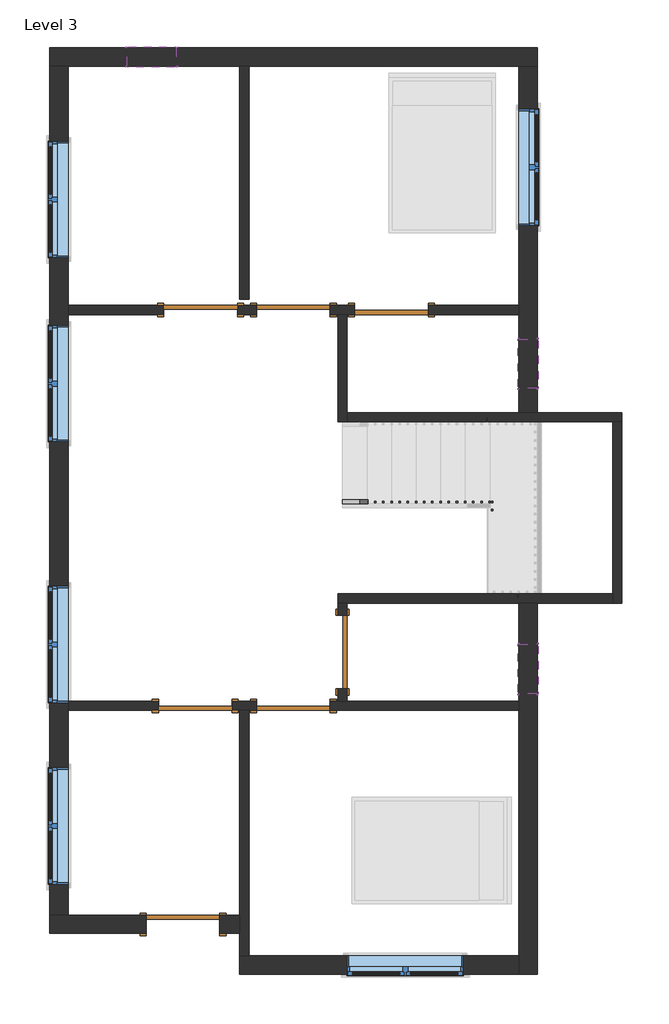
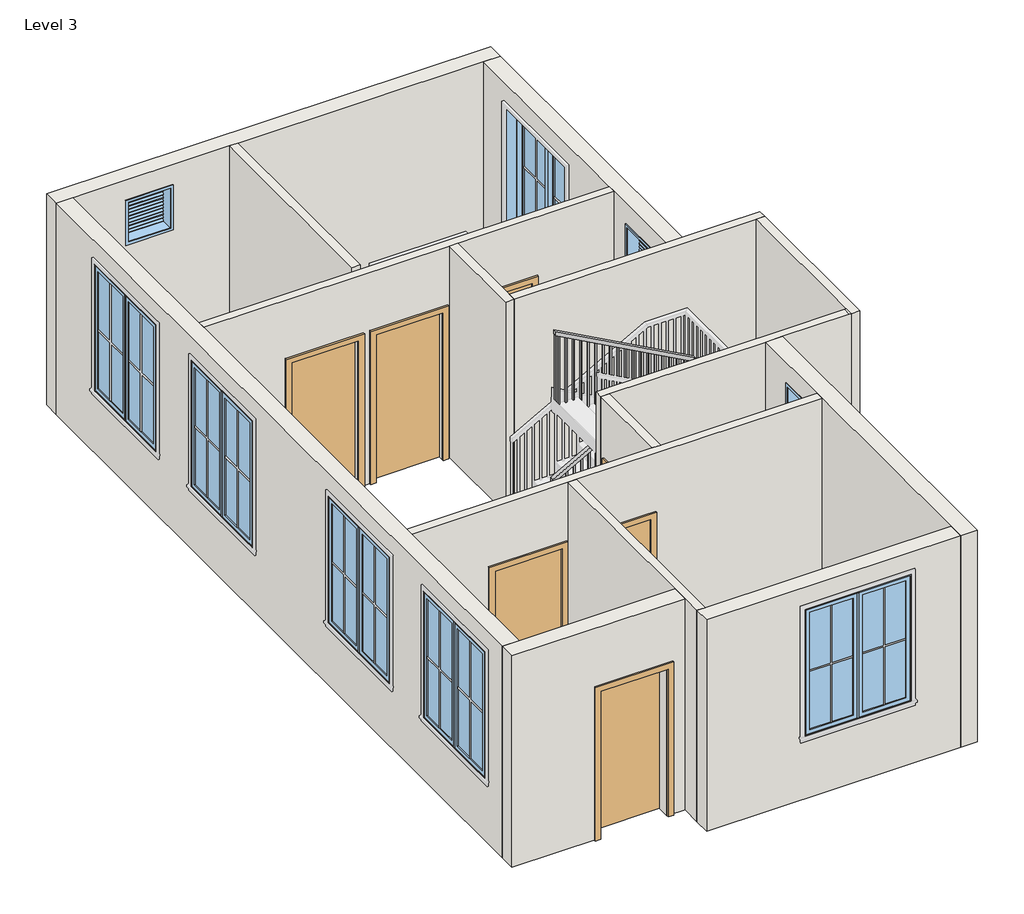
# One storey, part 1 of 2: 15 walls, 9 windows, 7 doors, 1 railing.
"""IFC4 building model written with IfcOpenShell, lengths in millimetres."""

from ifc_helpers import new_model, si_unit, frame, origin, place, context, project, spatial, polyline, outline, extrude, faceted_brep, transform, mapped, element, save
from components import door_e5f9f3c4, door_305aa2a5, door_0ca8825f, window_9ac97e1a, window_f2d8fef0

model = new_model("IFC4")

# Units and contexts
model_context = context("Model", 3, world=origin())
ifc_project = project(units=[si_unit("LENGTHUNIT", "METRE", prefix="MILLI")], contexts=[model_context])

# Site, building, storey
site = spatial("IfcSite", under=ifc_project)
building = spatial("IfcBuilding", under=site)
storey = spatial("IfcBuildingStorey", under=building, Name="Level 3", Elevation=3200.4)

# Doors
placement = place(None, origin())
door_shape = door_e5f9f3c4(model_context)
element("IfcDoor", 1, ObjectType="Single-Flush : 36\" x 84\"", at=placement, inside=storey, context=model_context, shape_type="MappedRepresentation", body=[
    mapped(door_shape, transform((-2929.7888307, 2238.9017201, 3200.4), x_axis=(1.0, 0.0, 0.0), y_axis=(0.0, 1.0, 0.0), z_axis=(0.0, 0.0, 1.0))),
])
element("IfcDoor", 2, ObjectType="Single-Flush : 36\" x 84\"", at=placement, inside=storey, context=model_context, shape_type="MappedRepresentation", body=[
    mapped(door_shape, transform((-558.0638307, 2238.9017201, 3200.4), x_axis=(-1.0, 0.0, 0.0), y_axis=(0.0, -1.0, 0.0), z_axis=(0.0, 0.0, 1.0))),
])
element("IfcDoor", 3, ObjectType="Single-Flush : 36\" x 84\"", at=placement, inside=storey, context=model_context, shape_type="MappedRepresentation", body=[
    mapped(door_shape, transform((-1167.6638307, -2009.2482799, 3200.4), x_axis=(0.0, -1.0, 0.0), y_axis=(1.0, 0.0, 0.0), z_axis=(0.0, 0.0, 1.0))),
])
element("IfcDoor", 4, ObjectType="Single-Flush : 36\" x 84\"", at=placement, inside=storey, context=model_context, shape_type="MappedRepresentation", body=[
    mapped(door_shape, transform((-1777.2638307, -2675.9982799, 3200.4), x_axis=(-1.0, 0.0, 0.0), y_axis=(0.0, -1.0, 0.0), z_axis=(0.0, 0.0, 1.0))),
])
door_2_shape = door_305aa2a5(model_context)
element("IfcDoor", 5, ObjectType="Single-Flush : 36\" x 84\"", at=placement, inside=storey, context=model_context, shape_type="MappedRepresentation", body=[
    mapped(door_2_shape, transform((-1777.2638307, 2238.9017201, 3200.4), x_axis=(-1.0, 0.0, 0.0), y_axis=(0.0, -1.0, 0.0), z_axis=(0.0, 0.0, 1.0))),
])
element("IfcDoor", 6, ObjectType="Single-Flush : 36\" x 84\"", at=placement, inside=storey, context=model_context, shape_type="MappedRepresentation", body=[
    mapped(door_2_shape, transform((-2996.4638307, -2675.9982799, 3200.4), x_axis=(1.0, 0.0, 0.0), y_axis=(0.0, 1.0, 0.0), z_axis=(0.0, 0.0, 1.0))),
])
door_3_shape = door_0ca8825f(model_context)
element("IfcDoor", 7, ObjectType="Single-Flush : 36\" x 84\"", at=placement, inside=storey, context=model_context, shape_type="MappedRepresentation", body=[
    mapped(door_3_shape, transform((-3148.8638307, -5387.4482799, 3200.4), x_axis=(1.0, 0.0, 0.0), y_axis=(0.0, 1.0, 0.0), z_axis=(0.0, 0.0, 1.0))),
])

# Railing
element("IfcRailing", 8, ObjectType="Handrail - Rectangular", at=placement, inside=storey, context=model_context, shape_type="SolidModel", body=[
    faceted_brep([(-1167.6638307, -116.9482799, 4284.1333333), (-1167.6638307, -116.9482799, 4226.0675836), (-1167.6638307, -167.7482799, 4226.0675836), (-1167.6638307, -167.7482799, 4284.1333333), (591.2861693, -116.9482799, 5257.9464821), (642.0861693, -116.9482799, 5228.0052998), (642.0861693, -167.7482799, 5228.0052998), (591.2861693, -167.7482799, 5257.9464821), (591.2861693, -116.9482799, 5300.1333333), (642.0861693, -116.9482799, 5249.3333333), (642.0861693, -167.7482799, 5249.3333333), (591.2861693, -167.7482799, 5300.1333333), (718.2861693, -116.9482799, 5300.1333333), (718.2861693, -116.9482799, 5249.3333333), (667.4861693, -167.7482799, 5249.3333333), (667.4861693, -167.7482799, 5300.1333333), (718.2861693, -218.5482799, 5300.1333333), (667.4861693, -218.5482799, 5300.1333333), (667.4861693, -269.3482799, 5249.3333333), (718.2861693, -269.3482799, 5249.3333333)], [[[0, 1, 2, 3]], [[1, 0, 4, 5]], [[2, 1, 5, 6]], [[3, 2, 6, 7]], [[0, 3, 7, 4]], [[5, 4, 8, 9]], [[6, 5, 9, 10]], [[7, 6, 10, 11]], [[4, 7, 11, 8]], [[9, 8, 12, 13]], [[10, 9, 13, 14]], [[11, 10, 14, 15]], [[8, 11, 15, 12]], [[16, 17, 18, 19]], [[13, 12, 16, 19]], [[14, 13, 19, 18]], [[15, 14, 18, 17]], [[12, 15, 17, 16]]]),
    faceted_brep([(718.2861693, -218.5482799, 5300.1333333), (718.2861693, -269.3482799, 5249.3333333), (667.4861693, -269.3482799, 5249.3333333), (667.4861693, -218.5482799, 5300.1333333), (718.2861693, -218.5482799, 5441.6310502), (667.4861693, -218.5482799, 5411.5403208), (667.4861693, -269.3482799, 5411.5403208), (718.2861693, -269.3482799, 5441.6310502)], [[[0, 1, 2, 3]], [[4, 5, 6, 7]], [[1, 0, 4, 7]], [[2, 1, 7, 6]], [[3, 2, 6, 5]], [[0, 3, 5, 4]]]),
    faceted_brep([(718.2861693, -269.3482799, 5441.6310502), (667.4861693, -269.3482799, 5411.5403208), (667.4861693, -218.5482799, 5411.5403208), (718.2861693, -218.5482799, 5441.6310502), (-1186.7138307, -269.3482799, 6485.4666667), (-1186.7138307, -218.5482799, 6485.4666667), (-1186.7138307, -218.5482799, 6427.5403208), (-1186.7138307, -269.3482799, 6427.5403208)], [[[0, 1, 2, 3]], [[4, 5, 6, 7]], [[1, 0, 4, 7]], [[2, 1, 7, 6]], [[3, 2, 6, 5]], [[0, 3, 5, 4]]]),
    extrude(outline(polyline([(6394.4855263, -1126.3888307), (6404.9238825, -1145.4388307), (5401.7333333, -1145.4388307), (5401.7333333, -1126.3888307), (6394.4855263, -1126.3888307)])), frame((0.0, -253.4732799, 0.0), z_axis=(0.0, 1.0, 0.0), x_axis=(0.0, 0.0, 1.0)), (0.0, 0.0, 1.0), 19.05),
    extrude(outline(polyline([(6338.8142934, -1024.7888307), (6349.2526496, -1043.8388307), (5401.7333333, -1043.8388307), (5401.7333333, -1024.7888307), (6338.8142934, -1024.7888307)])), frame((0.0, -253.4732799, 0.0), z_axis=(0.0, 1.0, 0.0), x_axis=(0.0, 0.0, 1.0)), (0.0, 0.0, 1.0), 19.05),
    extrude(outline(polyline([(6283.1430606, -923.1888307), (6293.5814167, -942.2388307), (5401.7333333, -942.2388307), (5401.7333333, -923.1888307), (6283.1430606, -923.1888307)])), frame((0.0, -253.4732799, 0.0), z_axis=(0.0, 1.0, 0.0), x_axis=(0.0, 0.0, 1.0)), (0.0, 0.0, 1.0), 19.05),
    extrude(outline(polyline([(6227.4718277, -821.5888307), (6237.9101838, -840.6388307), (5232.4, -840.6388307), (5232.4, -821.5888307), (6227.4718277, -821.5888307)])), frame((0.0, -253.4732799, 0.0), z_axis=(0.0, 1.0, 0.0), x_axis=(0.0, 0.0, 1.0)), (0.0, 0.0, 1.0), 19.05),
    extrude(outline(polyline([(6171.8005948, -719.9888307), (6182.238951, -739.0388307), (5232.4, -739.0388307), (5232.4, -719.9888307), (6171.8005948, -719.9888307)])), frame((0.0, -253.4732799, 0.0), z_axis=(0.0, 1.0, 0.0), x_axis=(0.0, 0.0, 1.0)), (0.0, 0.0, 1.0), 19.05),
    extrude(outline(polyline([(6116.1293619, -618.3888307), (6126.5677181, -637.4388307), (5232.4, -637.4388307), (5232.4, -618.3888307), (6116.1293619, -618.3888307)])), frame((0.0, -253.4732799, 0.0), z_axis=(0.0, 1.0, 0.0), x_axis=(0.0, 0.0, 1.0)), (0.0, 0.0, 1.0), 19.05),
    extrude(outline(polyline([(6060.458129, -516.7888307), (6070.8964852, -535.8388307), (5063.0666667, -535.8388307), (5063.0666667, -516.7888307), (6060.458129, -516.7888307)])), frame((0.0, -253.4732799, 0.0), z_axis=(0.0, 1.0, 0.0), x_axis=(0.0, 0.0, 1.0)), (0.0, 0.0, 1.0), 19.05),
    extrude(outline(polyline([(6004.7868962, -415.1888307), (6015.2252523, -434.2388307), (5063.0666667, -434.2388307), (5063.0666667, -415.1888307), (6004.7868962, -415.1888307)])), frame((0.0, -253.4732799, 0.0), z_axis=(0.0, 1.0, 0.0), x_axis=(0.0, 0.0, 1.0)), (0.0, 0.0, 1.0), 19.05),
    extrude(outline(polyline([(5949.1156633, -313.5888307), (5959.5540195, -332.6388307), (5063.0666667, -332.6388307), (5063.0666667, -313.5888307), (5949.1156633, -313.5888307)])), frame((0.0, -253.4732799, 0.0), z_axis=(0.0, 1.0, 0.0), x_axis=(0.0, 0.0, 1.0)), (0.0, 0.0, 1.0), 19.05),
    extrude(outline(polyline([(5893.4444304, -211.9888307), (5903.8827866, -231.0388307), (4893.7333333, -231.0388307), (4893.7333333, -211.9888307), (5893.4444304, -211.9888307)])), frame((0.0, -253.4732799, 0.0), z_axis=(0.0, 1.0, 0.0), x_axis=(0.0, 0.0, 1.0)), (0.0, 0.0, 1.0), 19.05),
    extrude(outline(polyline([(5837.7731975, -110.3888307), (5848.2115537, -129.4388307), (4893.7333333, -129.4388307), (4893.7333333, -110.3888307), (5837.7731975, -110.3888307)])), frame((0.0, -253.4732799, 0.0), z_axis=(0.0, 1.0, 0.0), x_axis=(0.0, 0.0, 1.0)), (0.0, 0.0, 1.0), 19.05),
    extrude(outline(polyline([(5782.1019647, -8.7888307), (5792.5403208, -27.8388307), (4893.7333333, -27.8388307), (4893.7333333, -8.7888307), (5782.1019647, -8.7888307)])), frame((0.0, -253.4732799, 0.0), z_axis=(0.0, 1.0, 0.0), x_axis=(0.0, 0.0, 1.0)), (0.0, 0.0, 1.0), 19.05),
    extrude(outline(polyline([(5726.4307318, 92.8111693), (5736.8690879, 73.7611693), (4724.4, 73.7611693), (4724.4, 92.8111693), (5726.4307318, 92.8111693)])), frame((0.0, -253.4732799, 0.0), z_axis=(0.0, 1.0, 0.0), x_axis=(0.0, 0.0, 1.0)), (0.0, 0.0, 1.0), 19.05),
    extrude(outline(polyline([(5670.7594989, 194.4111693), (5681.1978551, 175.3611693), (4724.4, 175.3611693), (4724.4, 194.4111693), (5670.7594989, 194.4111693)])), frame((0.0, -253.4732799, 0.0), z_axis=(0.0, 1.0, 0.0), x_axis=(0.0, 0.0, 1.0)), (0.0, 0.0, 1.0), 19.05),
    extrude(outline(polyline([(5615.088266, 296.0111693), (5625.5266222, 276.9611693), (4724.4, 276.9611693), (4724.4, 296.0111693), (5615.088266, 296.0111693)])), frame((0.0, -253.4732799, 0.0), z_axis=(0.0, 1.0, 0.0), x_axis=(0.0, 0.0, 1.0)), (0.0, 0.0, 1.0), 19.05),
    extrude(outline(polyline([(5559.4170332, 397.6111693), (5569.8553893, 378.5611693), (4555.0666667, 378.5611693), (4555.0666667, 397.6111693), (5559.4170332, 397.6111693)])), frame((0.0, -253.4732799, 0.0), z_axis=(0.0, 1.0, 0.0), x_axis=(0.0, 0.0, 1.0)), (0.0, 0.0, 1.0), 19.05),
    extrude(outline(polyline([(5503.7458003, 499.2111693), (5514.1841564, 480.1611693), (4555.0666667, 480.1611693), (4555.0666667, 499.2111693), (5503.7458003, 499.2111693)])), frame((0.0, -253.4732799, 0.0), z_axis=(0.0, 1.0, 0.0), x_axis=(0.0, 0.0, 1.0)), (0.0, 0.0, 1.0), 19.05),
    extrude(outline(polyline([(5448.0745674, 600.8111693), (5458.5129236, 581.7611693), (4555.0666667, 581.7611693), (4555.0666667, 600.8111693), (5448.0745674, 600.8111693)])), frame((0.0, -253.4732799, 0.0), z_axis=(0.0, 1.0, 0.0), x_axis=(0.0, 0.0, 1.0)), (0.0, 0.0, 1.0), 19.05),
    extrude(outline(polyline([(651.6111693, -151.8732799), (651.6111693, -132.8232799), (670.6611693, -132.8232799), (670.6611693, -151.8732799), (651.6111693, -151.8732799)])), frame((0.0, 0.0, 4216.4), z_axis=(0.0, 0.0, 1.0), x_axis=(1.0, 0.0, 0.0)), (0.0, 0.0, 1.0), 1032.9333333),
    extrude(outline(polyline([(5187.5762341, 569.0611693), (5177.0295213, 550.0111693), (4216.4, 550.0111693), (4216.4, 569.0611693), (5187.5762341, 569.0611693)])), frame((0.0, -151.8732799, 0.0), z_axis=(0.0, 1.0, 0.0), x_axis=(0.0, 0.0, 1.0)), (0.0, 0.0, 1.0), 19.05),
    extrude(outline(polyline([(5131.3270991, 467.4611693), (5120.7803863, 448.4111693), (4216.4, 448.4111693), (4216.4, 467.4611693), (5131.3270991, 467.4611693)])), frame((0.0, -151.8732799, 0.0), z_axis=(0.0, 1.0, 0.0), x_axis=(0.0, 0.0, 1.0)), (0.0, 0.0, 1.0), 19.05),
    extrude(outline(polyline([(5075.0779642, 365.8611693), (5064.5312514, 346.8111693), (4047.0666667, 346.8111693), (4047.0666667, 365.8611693), (5075.0779642, 365.8611693)])), frame((0.0, -151.8732799, 0.0), z_axis=(0.0, 1.0, 0.0), x_axis=(0.0, 0.0, 1.0)), (0.0, 0.0, 1.0), 19.05),
    extrude(outline(polyline([(5018.8288292, 264.2611693), (5008.2821164, 245.2111693), (4047.0666667, 245.2111693), (4047.0666667, 264.2611693), (5018.8288292, 264.2611693)])), frame((0.0, -151.8732799, 0.0), z_axis=(0.0, 1.0, 0.0), x_axis=(0.0, 0.0, 1.0)), (0.0, 0.0, 1.0), 19.05),
    extrude(outline(polyline([(4962.5796943, 162.6611693), (4952.0329815, 143.6111693), (4047.0666667, 143.6111693), (4047.0666667, 162.6611693), (4962.5796943, 162.6611693)])), frame((0.0, -151.8732799, 0.0), z_axis=(0.0, 1.0, 0.0), x_axis=(0.0, 0.0, 1.0)), (0.0, 0.0, 1.0), 19.05),
    extrude(outline(polyline([(4906.3305593, 61.0611693), (4895.7838465, 42.0111693), (3877.7333333, 42.0111693), (3877.7333333, 61.0611693), (4906.3305593, 61.0611693)])), frame((0.0, -151.8732799, 0.0), z_axis=(0.0, 1.0, 0.0), x_axis=(0.0, 0.0, 1.0)), (0.0, 0.0, 1.0), 19.05),
    extrude(outline(polyline([(4850.0814244, -40.5388307), (4839.5347116, -59.5888307), (3877.7333333, -59.5888307), (3877.7333333, -40.5388307), (4850.0814244, -40.5388307)])), frame((0.0, -151.8732799, 0.0), z_axis=(0.0, 1.0, 0.0), x_axis=(0.0, 0.0, 1.0)), (0.0, 0.0, 1.0), 19.05),
    extrude(outline(polyline([(4793.8322895, -142.1388307), (4783.2855766, -161.1888307), (3877.7333333, -161.1888307), (3877.7333333, -142.1388307), (4793.8322895, -142.1388307)])), frame((0.0, -151.8732799, 0.0), z_axis=(0.0, 1.0, 0.0), x_axis=(0.0, 0.0, 1.0)), (0.0, 0.0, 1.0), 19.05),
    extrude(outline(polyline([(4737.5831545, -243.7388307), (4727.0364417, -262.7888307), (3708.4, -262.7888307), (3708.4, -243.7388307), (4737.5831545, -243.7388307)])), frame((0.0, -151.8732799, 0.0), z_axis=(0.0, 1.0, 0.0), x_axis=(0.0, 0.0, 1.0)), (0.0, 0.0, 1.0), 19.05),
    extrude(outline(polyline([(4681.3340196, -345.3388307), (4670.7873068, -364.3888307), (3708.4, -364.3888307), (3708.4, -345.3388307), (4681.3340196, -345.3388307)])), frame((0.0, -151.8732799, 0.0), z_axis=(0.0, 1.0, 0.0), x_axis=(0.0, 0.0, 1.0)), (0.0, 0.0, 1.0), 19.05),
    extrude(outline(polyline([(4625.0848846, -446.9388307), (4614.5381718, -465.9888307), (3708.4, -465.9888307), (3708.4, -446.9388307), (4625.0848846, -446.9388307)])), frame((0.0, -151.8732799, 0.0), z_axis=(0.0, 1.0, 0.0), x_axis=(0.0, 0.0, 1.0)), (0.0, 0.0, 1.0), 19.05),
    extrude(outline(polyline([(4568.8357497, -548.5388307), (4558.2890369, -567.5888307), (3539.0666667, -567.5888307), (3539.0666667, -548.5388307), (4568.8357497, -548.5388307)])), frame((0.0, -151.8732799, 0.0), z_axis=(0.0, 1.0, 0.0), x_axis=(0.0, 0.0, 1.0)), (0.0, 0.0, 1.0), 19.05),
    extrude(outline(polyline([(4512.5866147, -650.1388307), (4502.0399019, -669.1888307), (3539.0666667, -669.1888307), (3539.0666667, -650.1388307), (4512.5866147, -650.1388307)])), frame((0.0, -151.8732799, 0.0), z_axis=(0.0, 1.0, 0.0), x_axis=(0.0, 0.0, 1.0)), (0.0, 0.0, 1.0), 19.05),
    extrude(outline(polyline([(4456.3374798, -751.7388307), (4445.790767, -770.7888307), (3539.0666667, -770.7888307), (3539.0666667, -751.7388307), (4456.3374798, -751.7388307)])), frame((0.0, -151.8732799, 0.0), z_axis=(0.0, 1.0, 0.0), x_axis=(0.0, 0.0, 1.0)), (0.0, 0.0, 1.0), 19.05),
    extrude(outline(polyline([(4400.0883448, -853.3388307), (4389.541632, -872.3888307), (3369.7333333, -872.3888307), (3369.7333333, -853.3388307), (4400.0883448, -853.3388307)])), frame((0.0, -151.8732799, 0.0), z_axis=(0.0, 1.0, 0.0), x_axis=(0.0, 0.0, 1.0)), (0.0, 0.0, 1.0), 19.05),
    extrude(outline(polyline([(4343.8392099, -954.9388307), (4333.2924971, -973.9888307), (3369.7333333, -973.9888307), (3369.7333333, -954.9388307), (4343.8392099, -954.9388307)])), frame((0.0, -151.8732799, 0.0), z_axis=(0.0, 1.0, 0.0), x_axis=(0.0, 0.0, 1.0)), (0.0, 0.0, 1.0), 19.05),
    extrude(outline(polyline([(4287.5900749, -1056.5388307), (4277.0433621, -1075.5888307), (3369.7333333, -1075.5888307), (3369.7333333, -1056.5388307), (4287.5900749, -1056.5388307)])), frame((0.0, -151.8732799, 0.0), z_axis=(0.0, 1.0, 0.0), x_axis=(0.0, 0.0, 1.0)), (0.0, 0.0, 1.0), 19.05),
    extrude(outline(polyline([(683.3611693, -234.4232799), (702.4111693, -234.4232799), (702.4111693, -253.4732799), (683.3611693, -253.4732799), (683.3611693, -234.4232799)])), frame((0.0, 0.0, 4385.7333333), z_axis=(0.0, 0.0, 1.0), x_axis=(1.0, 0.0, 0.0)), (0.0, 0.0, 1.0), 863.6),
    extrude(outline(polyline([(683.3611693, -151.8732799), (683.3611693, -132.8232799), (702.4111693, -132.8232799), (702.4111693, -151.8732799), (683.3611693, -151.8732799)])), frame((0.0, 0.0, 4385.7333333), z_axis=(0.0, 0.0, 1.0), x_axis=(1.0, 0.0, 0.0)), (0.0, 0.0, 1.0), 863.6),
    extrude(outline(polyline([(6417.1019647, -1167.6638307), (6427.5403208, -1186.7138307), (5401.7333333, -1186.7138307), (5401.7333333, -1167.6638307), (6417.1019647, -1167.6638307)])), frame((0.0, -253.4732799, 0.0), z_axis=(0.0, 1.0, 0.0), x_axis=(0.0, 0.0, 1.0)), (0.0, 0.0, 1.0), 19.05),
    extrude(outline(polyline([(4236.6142964, -1148.6138307), (4226.0675836, -1167.6638307), (3369.7333333, -1167.6638307), (3369.7333333, -1148.6138307), (4236.6142964, -1148.6138307)])), frame((0.0, -151.8732799, 0.0), z_axis=(0.0, 1.0, 0.0), x_axis=(0.0, 0.0, 1.0)), (0.0, 0.0, 1.0), 19.05),
])

# Walls
element("IfcWall", 9, ObjectType="WALL 4.5\"", at=placement, inside=storey, context=model_context, shape_type="SweptSolid", body=[
    extrude(outline(polyline([(-2444.0138307, 2372.2517201), (-2444.0138307, 5267.8517201), (-2329.7138307, 5267.8517201), (-2329.7138307, 2372.2517201), (-2444.0138307, 2372.2517201)])), frame((0.0, 0.0, 3200.4), z_axis=(0.0, 0.0, 1.0), x_axis=(1.0, 0.0, 0.0)), (0.0, 0.0, 1.0), 3048.0),
])
element("IfcWall", 10, ObjectType="WALL 4.5\"", at=placement, inside=storey, context=model_context, shape_type="Brep", body=[
    faceted_brep([(-1320.0638307, 2181.7517201, 3200.4), (-1224.8138307, 2181.7517201, 3200.4), (-1110.5138307, 2181.7517201, 3200.4), (-1015.2638307, 2181.7517201, 3200.4), (-1015.2638307, 2181.7517201, 5334.0), (-100.8638307, 2181.7517201, 5334.0), (-100.8638307, 2181.7517201, 3200.4), (1023.0861693, 2181.7517201, 3200.4), (1023.0861693, 2181.7517201, 6248.4), (-1110.5138307, 2181.7517201, 6248.4), (-1224.8138307, 2181.7517201, 6248.4), (-4577.6138307, 2181.7517201, 6248.4), (-4577.6138307, 2181.7517201, 3200.4), (-3386.9888307, 2181.7517201, 3200.4), (-3386.9888307, 2181.7517201, 5334.0), (-2472.5888307, 2181.7517201, 5334.0), (-2472.5888307, 2181.7517201, 3200.4), (-2234.4638307, 2181.7517201, 3200.4), (-2234.4638307, 2181.7517201, 5334.0), (-1320.0638307, 2181.7517201, 5334.0), (-1015.2638307, 2296.0517201, 5334.0), (-1015.2638307, 2296.0517201, 3200.4), (-1320.0638307, 2296.0517201, 3200.4), (-1320.0638307, 2296.0517201, 5334.0), (-2234.4638307, 2296.0517201, 5334.0), (-2234.4638307, 2296.0517201, 3200.4), (-2472.5888307, 2296.0517201, 3200.4), (-2472.5888307, 2296.0517201, 5334.0), (-3386.9888307, 2296.0517201, 5334.0), (-3386.9888307, 2296.0517201, 3200.4), (-4577.6138307, 2296.0517201, 3200.4), (-4577.6138307, 2296.0517201, 6248.4), (1023.0861693, 2296.0517201, 6248.4), (1023.0861693, 2296.0517201, 3200.4), (-100.8638307, 2296.0517201, 3200.4), (-100.8638307, 2296.0517201, 5334.0)], [[[0, 1, 2, 3, 4, 5, 6, 7, 8, 9, 10, 11, 12, 13, 14, 15, 16, 17, 18, 19]], [[20, 21, 22, 23, 24, 25, 26, 27, 28, 29, 30, 31, 32, 33, 34, 35]], [[13, 12, 30, 29]], [[26, 25, 17, 16]], [[34, 33, 7, 6]], [[22, 21, 3, 2, 1, 0]], [[8, 7, 33, 32]], [[12, 11, 31, 30]], [[27, 26, 16, 15]], [[28, 27, 15, 14]], [[29, 28, 14, 13]], [[18, 17, 25, 24]], [[19, 18, 24, 23]], [[0, 19, 23, 22]], [[4, 3, 21, 20]], [[5, 4, 20, 35]], [[6, 5, 35, 34]], [[11, 10, 9, 8, 32, 31]]]),
])
element("IfcWall", 11, ObjectType="WALL 4.5\"", at=placement, inside=storey, context=model_context, shape_type="Brep", body=[
    faceted_brep([(-1224.8138307, 2181.7517201, 3200.4), (-1224.8138307, 848.2517201, 3200.4), (-1224.8138307, 848.2517201, 6248.4), (-1224.8138307, 2181.7517201, 6248.4), (-1110.5138307, 2181.7517201, 3200.4), (-1110.5138307, 2181.7517201, 6248.4), (-1110.5138307, 962.5517201, 6248.4), (-1110.5138307, 848.2517201, 6248.4), (-1110.5138307, 848.2517201, 3200.4), (-1110.5138307, 962.5517201, 3200.4)], [[[0, 1, 2, 3]], [[4, 5, 6, 7, 8, 9]], [[1, 0, 4, 9, 8]], [[0, 3, 5, 4]], [[2, 1, 8, 7]], [[3, 2, 7, 6, 5]]]),
])
element("IfcWall", 12, ObjectType="WALL 4.5\"", at=placement, inside=storey, context=model_context, shape_type="Brep", body=[
    faceted_brep([(-1110.5138307, 848.2517201, 3200.4), (2191.4861693, 848.2517201, 3200.4), (2305.7861693, 848.2517201, 3200.4), (2305.7861693, 848.2517201, 6248.4), (2191.4861693, 848.2517201, 6248.4), (-1110.5138307, 848.2517201, 6248.4), (-1110.5138307, 962.5517201, 3200.4), (-1110.5138307, 962.5517201, 6248.4), (1023.0861693, 962.5517201, 6248.4), (1251.6861693, 962.5517201, 6248.4), (2305.7861693, 962.5517201, 6248.4), (2305.7861693, 962.5517201, 3200.4), (1251.6861693, 962.5517201, 3200.4), (1023.0861693, 962.5517201, 3200.4)], [[[0, 1, 2, 3, 4, 5]], [[6, 7, 8, 9, 10, 11, 12, 13]], [[2, 1, 0, 6, 13, 12, 11]], [[5, 4, 3, 10, 9, 8, 7]], [[0, 5, 7, 6]], [[3, 2, 11, 10]]]),
])
element("IfcWall", 13, ObjectType="WALL 4.5\"", at=placement, inside=storey, context=model_context, shape_type="Brep", body=[
    faceted_brep([(2191.4861693, 848.2517201, 3200.4), (2191.4861693, -1285.3482799, 3200.4), (2191.4861693, -1399.6482799, 3200.4), (2191.4861693, -1399.6482799, 6248.4), (2191.4861693, -1285.3482799, 6248.4), (2191.4861693, 848.2517201, 6248.4), (2305.7861693, 848.2517201, 3200.4), (2305.7861693, 848.2517201, 6248.4), (2305.7861693, -1399.6482799, 6248.4), (2305.7861693, -1399.6482799, 3200.4)], [[[0, 1, 2, 3, 4, 5]], [[6, 7, 8, 9]], [[2, 1, 0, 6, 9]], [[5, 4, 3, 8, 7]], [[0, 5, 7, 6]], [[3, 2, 9, 8]]]),
])
element("IfcWall", 14, ObjectType="WALL 4.5\"", at=placement, inside=storey, context=model_context, shape_type="Brep", body=[
    faceted_brep([(2191.4861693, -1285.3482799, 3200.4), (-1224.8138307, -1285.3482799, 3200.4), (-1224.8138307, -1285.3482799, 6248.4), (-881.9138307, -1285.3482799, 6248.4), (1251.6861693, -1285.3482799, 6248.4), (2166.0861693, -1285.3482799, 6248.4), (2191.4861693, -1285.3482799, 6248.4), (2191.4861693, -1399.6482799, 3200.4), (2191.4861693, -1399.6482799, 6248.4), (2166.0861693, -1399.6482799, 6248.4), (1251.6861693, -1399.6482799, 6248.4), (1023.0861693, -1399.6482799, 6248.4), (-1110.5138307, -1399.6482799, 6248.4), (-1224.8138307, -1399.6482799, 6248.4), (-1224.8138307, -1399.6482799, 3200.4), (-1110.5138307, -1399.6482799, 3200.4), (1023.0861693, -1399.6482799, 3200.4), (1251.6861693, -1399.6482799, 3200.4)], [[[0, 1, 2, 3, 4, 5, 6]], [[7, 8, 9, 10, 11, 12, 13, 14, 15, 16, 17]], [[1, 0, 7, 17, 16, 15, 14]], [[0, 6, 8, 7]], [[2, 1, 14, 13]], [[6, 5, 9, 8]], [[5, 4, 3, 2, 13, 12, 11, 10, 9]]]),
])
element("IfcWall", 15, ObjectType="WALL 4.5\"", at=placement, inside=storey, context=model_context, shape_type="SweptSolid", body=[
    extrude(outline(polyline([(-2466.4482799, 5334.0), (-2466.4482799, 3200.4), (-2618.8482799, 3200.4), (-2618.8482799, 6248.4), (-1399.6482799, 6248.4), (-1399.6482799, 3200.4), (-1552.0482799, 3200.4), (-1552.0482799, 5334.0), (-2466.4482799, 5334.0)])), frame((-1224.8138307, 0.0, 0.0), z_axis=(1.0, 0.0, 0.0), x_axis=(0.0, 1.0, 0.0)), (0.0, 0.0, 1.0), 114.3),
])
element("IfcWall", 16, ObjectType="WALL 4.5\"", at=placement, inside=storey, context=model_context, shape_type="Brep", body=[
    faceted_brep([(-2234.4638307, -2618.8482799, 3200.4), (-2539.2638307, -2618.8482799, 3200.4), (-2539.2638307, -2618.8482799, 5334.0), (-3453.6638307, -2618.8482799, 5334.0), (-3453.6638307, -2618.8482799, 3200.4), (-4577.6138307, -2618.8482799, 3200.4), (-4577.6138307, -2618.8482799, 6248.4), (-1224.8138307, -2618.8482799, 6248.4), (-1110.5138307, -2618.8482799, 6248.4), (1023.0861693, -2618.8482799, 6248.4), (1023.0861693, -2618.8482799, 3200.4), (-1110.5138307, -2618.8482799, 3200.4), (-1224.8138307, -2618.8482799, 3200.4), (-1320.0638307, -2618.8482799, 3200.4), (-1320.0638307, -2618.8482799, 5334.0), (-2234.4638307, -2618.8482799, 5334.0), (-2539.2638307, -2733.1482799, 5334.0), (-2539.2638307, -2733.1482799, 3200.4), (-2444.0138307, -2733.1482799, 3200.4), (-2329.7138307, -2733.1482799, 3200.4), (-2234.4638307, -2733.1482799, 3200.4), (-2234.4638307, -2733.1482799, 5334.0), (-1320.0638307, -2733.1482799, 5334.0), (-1320.0638307, -2733.1482799, 3200.4), (1023.0861693, -2733.1482799, 3200.4), (1023.0861693, -2733.1482799, 6248.4), (-2329.7138307, -2733.1482799, 6248.4), (-2444.0138307, -2733.1482799, 6248.4), (-4577.6138307, -2733.1482799, 6248.4), (-4577.6138307, -2733.1482799, 3200.4), (-3453.6638307, -2733.1482799, 3200.4), (-3453.6638307, -2733.1482799, 5334.0)], [[[0, 1, 2, 3, 4, 5, 6, 7, 8, 9, 10, 11, 12, 13, 14, 15]], [[16, 17, 18, 19, 20, 21, 22, 23, 24, 25, 26, 27, 28, 29, 30, 31]], [[13, 12, 11, 10, 24, 23]], [[30, 29, 5, 4]], [[20, 19, 18, 17, 1, 0]], [[10, 9, 25, 24]], [[6, 5, 29, 28]], [[21, 20, 0, 15]], [[22, 21, 15, 14]], [[23, 22, 14, 13]], [[2, 1, 17, 16]], [[3, 2, 16, 31]], [[4, 3, 31, 30]], [[9, 8, 7, 6, 28, 27, 26, 25]]]),
])
element("IfcWall", 17, ObjectType="WALL 4.5\"", at=placement, inside=storey, context=model_context, shape_type="Brep", body=[
    faceted_brep([(-2329.7138307, -5781.1482799, 3200.4), (-2329.7138307, -2733.1482799, 3200.4), (-2329.7138307, -2733.1482799, 6248.4), (-2329.7138307, -5781.1482799, 6248.4), (-2444.0138307, -5781.1482799, 3200.4), (-2444.0138307, -5781.1482799, 6248.4), (-2444.0138307, -5501.7482799, 6248.4), (-2444.0138307, -5273.1482799, 6248.4), (-2444.0138307, -2733.1482799, 6248.4), (-2444.0138307, -2733.1482799, 3200.4), (-2444.0138307, -5273.1482799, 3200.4), (-2444.0138307, -5501.7482799, 3200.4)], [[[0, 1, 2, 3]], [[4, 5, 6, 7, 8, 9, 10, 11]], [[1, 0, 4, 11, 10, 9]], [[0, 3, 5, 4]], [[2, 1, 9, 8]], [[3, 2, 8, 7, 6, 5]]]),
])
element("IfcWall", 18, ObjectType="WALL 9\"", at=placement, inside=storey, context=model_context, shape_type="Brep", body=[
    faceted_brep([(-4806.2138307, 5267.8517201, 3200.4), (-4577.6138307, 5267.8517201, 3200.4), (-2444.0138307, 5267.8517201, 3200.4), (-2329.7138307, 5267.8517201, 3200.4), (1023.0861693, 5267.8517201, 3200.4), (1251.6861693, 5267.8517201, 3200.4), (1251.6861693, 5267.8517201, 6248.4), (1023.0861693, 5267.8517201, 6248.4), (-2329.7138307, 5267.8517201, 6248.4), (-2444.0138307, 5267.8517201, 6248.4), (-4577.6138307, 5267.8517201, 6248.4), (-4806.2138307, 5267.8517201, 6248.4), (-3844.1888307, 5267.8517201, 5943.6), (-3234.5888307, 5267.8517201, 5943.6), (-3234.5888307, 5267.8517201, 5334.0), (-3844.1888307, 5267.8517201, 5334.0), (-4806.2138307, 5496.4517201, 3200.4), (-4806.2138307, 5496.4517201, 6248.4), (1251.6861693, 5496.4517201, 6248.4), (1251.6861693, 5496.4517201, 3200.4), (-3844.1888307, 5496.4517201, 5943.6), (-3844.1888307, 5496.4517201, 5334.0), (-3234.5888307, 5496.4517201, 5334.0), (-3234.5888307, 5496.4517201, 5943.6)], [[[0, 1, 2, 3, 4, 5, 6, 7, 8, 9, 10, 11], [12, 13, 14, 15]], [[16, 17, 18, 19], [20, 21, 22, 23]], [[5, 4, 3, 2, 1, 0, 16, 19]], [[6, 5, 19, 18]], [[0, 11, 17, 16]], [[21, 20, 12, 15]], [[22, 21, 15, 14]], [[23, 22, 14, 13]], [[20, 23, 13, 12]], [[11, 10, 9, 8, 7, 6, 18, 17]]]),
])
element("IfcWall", 19, ObjectType="WALL 9\"", at=placement, inside=storey, context=model_context, shape_type="Brep", body=[
    faceted_brep([(1023.0861693, 5267.8517201, 3200.4), (1023.0861693, 2296.0517201, 3200.4), (1023.0861693, 2181.7517201, 3200.4), (1023.0861693, 962.5517201, 3200.4), (1023.0861693, 962.5517201, 6248.4), (1023.0861693, 2181.7517201, 6248.4), (1023.0861693, 2296.0517201, 6248.4), (1023.0861693, 5267.8517201, 6248.4), (1023.0861693, 3286.6517201, 5943.6), (1023.0861693, 3286.6517201, 4114.8), (1023.0861693, 4734.4517201, 4114.8), (1023.0861693, 4734.4517201, 5943.6), (1023.0861693, 1876.9517201, 5943.6), (1023.0861693, 1267.3517201, 5943.6), (1023.0861693, 1267.3517201, 5334.0), (1023.0861693, 1876.9517201, 5334.0), (1251.6861693, 5267.8517201, 3200.4), (1251.6861693, 5267.8517201, 6248.4), (1251.6861693, 962.5517201, 6248.4), (1251.6861693, 962.5517201, 3200.4), (1251.6861693, 3286.6517201, 5943.6), (1251.6861693, 4734.4517201, 5943.6), (1251.6861693, 4734.4517201, 4114.8), (1251.6861693, 3286.6517201, 4114.8), (1251.6861693, 1876.9517201, 5943.6), (1251.6861693, 1876.9517201, 5334.0), (1251.6861693, 1267.3517201, 5334.0), (1251.6861693, 1267.3517201, 5943.6)], [[[0, 1, 2, 3, 4, 5, 6, 7], [8, 9, 10, 11], [12, 13, 14, 15]], [[16, 17, 18, 19], [20, 21, 22, 23], [24, 25, 26, 27]], [[3, 2, 1, 0, 16, 19]], [[0, 7, 17, 16]], [[4, 3, 19, 18]], [[9, 8, 20, 23]], [[10, 9, 23, 22]], [[11, 10, 22, 21]], [[8, 11, 21, 20]], [[25, 24, 12, 15]], [[26, 25, 15, 14]], [[27, 26, 14, 13]], [[24, 27, 13, 12]], [[7, 6, 5, 4, 18, 17]]]),
])
element("IfcWall", 20, ObjectType="WALL 9\"", at=placement, inside=storey, context=model_context, shape_type="Brep", body=[
    faceted_brep([(1023.0861693, -1399.6482799, 3200.4), (1023.0861693, -2618.8482799, 3200.4), (1023.0861693, -2733.1482799, 3200.4), (1023.0861693, -5781.1482799, 3200.4), (1023.0861693, -6009.7482799, 3200.4), (1023.0861693, -6009.7482799, 6248.4), (1023.0861693, -5781.1482799, 6248.4), (1023.0861693, -2733.1482799, 6248.4), (1023.0861693, -2618.8482799, 6248.4), (1023.0861693, -1399.6482799, 6248.4), (1023.0861693, -1913.9982799, 5943.6), (1023.0861693, -2523.5982799, 5943.6), (1023.0861693, -2523.5982799, 5334.0), (1023.0861693, -1913.9982799, 5334.0), (1251.6861693, -1399.6482799, 3200.4), (1251.6861693, -1399.6482799, 6248.4), (1251.6861693, -6009.7482799, 6248.4), (1251.6861693, -6009.7482799, 3200.4), (1251.6861693, -1913.9982799, 5943.6), (1251.6861693, -1913.9982799, 5334.0), (1251.6861693, -2523.5982799, 5334.0), (1251.6861693, -2523.5982799, 5943.6)], [[[0, 1, 2, 3, 4, 5, 6, 7, 8, 9], [10, 11, 12, 13]], [[14, 15, 16, 17], [18, 19, 20, 21]], [[4, 3, 2, 1, 0, 14, 17]], [[5, 4, 17, 16]], [[0, 9, 15, 14]], [[19, 18, 10, 13]], [[20, 19, 13, 12]], [[21, 20, 12, 11]], [[18, 21, 11, 10]], [[9, 8, 7, 6, 5, 16, 15]]]),
])
element("IfcWall", 21, ObjectType="WALL 9\"", at=placement, inside=storey, context=model_context, shape_type="Brep", body=[
    faceted_brep([(1023.0861693, -5781.1482799, 3200.4), (-2329.7138307, -5781.1482799, 3200.4), (-2444.0138307, -5781.1482799, 3200.4), (-2444.0138307, -5781.1482799, 6248.4), (-2329.7138307, -5781.1482799, 6248.4), (1023.0861693, -5781.1482799, 6248.4), (-1110.5138307, -5781.1482799, 5943.6), (-1110.5138307, -5781.1482799, 4114.8), (337.2861693, -5781.1482799, 4114.8), (337.2861693, -5781.1482799, 5943.6), (1023.0861693, -6009.7482799, 3200.4), (1023.0861693, -6009.7482799, 6248.4), (-2444.0138307, -6009.7482799, 6248.4), (-2444.0138307, -6009.7482799, 3200.4), (-1110.5138307, -6009.7482799, 5943.6), (337.2861693, -6009.7482799, 5943.6), (337.2861693, -6009.7482799, 4114.8), (-1110.5138307, -6009.7482799, 4114.8)], [[[0, 1, 2, 3, 4, 5], [6, 7, 8, 9]], [[10, 11, 12, 13], [14, 15, 16, 17]], [[2, 1, 0, 10, 13]], [[0, 5, 11, 10]], [[3, 2, 13, 12]], [[7, 6, 14, 17]], [[8, 7, 17, 16]], [[9, 8, 16, 15]], [[6, 9, 15, 14]], [[5, 4, 3, 12, 11]]]),
])
element("IfcWall", 22, ObjectType="WALL 9\"", at=placement, inside=storey, context=model_context, shape_type="Brep", body=[
    faceted_brep([(-2691.6638307, -5501.7482799, 5334.0), (-2691.6638307, -5501.7482799, 3200.4), (-2444.0138307, -5501.7482799, 3200.4), (-2444.0138307, -5501.7482799, 6248.4), (-4806.2138307, -5501.7482799, 6248.4), (-4806.2138307, -5501.7482799, 3200.4), (-3606.0638307, -5501.7482799, 3200.4), (-3606.0638307, -5501.7482799, 5334.0), (-2444.0138307, -5273.1482799, 3200.4), (-2691.6638307, -5273.1482799, 3200.4), (-2691.6638307, -5273.1482799, 5334.0), (-3606.0638307, -5273.1482799, 5334.0), (-3606.0638307, -5273.1482799, 3200.4), (-4577.6138307, -5273.1482799, 3200.4), (-4806.2138307, -5273.1482799, 3200.4), (-4806.2138307, -5273.1482799, 6248.4), (-4577.6138307, -5273.1482799, 6248.4), (-2444.0138307, -5273.1482799, 6248.4)], [[[0, 1, 2, 3, 4, 5, 6, 7]], [[8, 9, 10, 11, 12, 13, 14, 15, 16, 17]], [[6, 5, 14, 13, 12]], [[2, 1, 9, 8]], [[5, 4, 15, 14]], [[3, 2, 8, 17]], [[10, 9, 1, 0]], [[11, 10, 0, 7]], [[12, 11, 7, 6]], [[4, 3, 17, 16, 15]]]),
])
element("IfcWall", 23, ObjectType="WALL 9\"", at=placement, inside=storey, context=model_context, shape_type="Brep", body=[
    faceted_brep([(-4577.6138307, -5273.1482799, 3200.4), (-4577.6138307, -2733.1482799, 3200.4), (-4577.6138307, -2618.8482799, 3200.4), (-4577.6138307, 2181.7517201, 3200.4), (-4577.6138307, 2296.0517201, 3200.4), (-4577.6138307, 5267.8517201, 3200.4), (-4577.6138307, 5267.8517201, 6248.4), (-4577.6138307, 2296.0517201, 6248.4), (-4577.6138307, 2181.7517201, 6248.4), (-4577.6138307, -2618.8482799, 6248.4), (-4577.6138307, -2733.1482799, 6248.4), (-4577.6138307, -5273.1482799, 6248.4), (-4577.6138307, -3444.3482799, 5943.6), (-4577.6138307, -3444.3482799, 4114.8), (-4577.6138307, -4892.1482799, 4114.8), (-4577.6138307, -4892.1482799, 5943.6), (-4577.6138307, -1190.0982799, 5943.6), (-4577.6138307, -1190.0982799, 4114.8), (-4577.6138307, -2637.8982799, 4114.8), (-4577.6138307, -2637.8982799, 5943.6), (-4577.6138307, 4334.4017201, 5943.6), (-4577.6138307, 4334.4017201, 4114.8), (-4577.6138307, 2886.6017201, 4114.8), (-4577.6138307, 2886.6017201, 5943.6), (-4577.6138307, 2048.4017201, 5943.6), (-4577.6138307, 2048.4017201, 4114.8), (-4577.6138307, 600.6017201, 4114.8), (-4577.6138307, 600.6017201, 5943.6), (-4806.2138307, -5273.1482799, 3200.4), (-4806.2138307, -5273.1482799, 6248.4), (-4806.2138307, 5267.8517201, 6248.4), (-4806.2138307, 5267.8517201, 3200.4), (-4806.2138307, -3444.3482799, 5943.6), (-4806.2138307, -4892.1482799, 5943.6), (-4806.2138307, -4892.1482799, 4114.8), (-4806.2138307, -3444.3482799, 4114.8), (-4806.2138307, -1190.0982799, 5943.6), (-4806.2138307, -2637.8982799, 5943.6), (-4806.2138307, -2637.8982799, 4114.8), (-4806.2138307, -1190.0982799, 4114.8), (-4806.2138307, 4334.4017201, 5943.6), (-4806.2138307, 2886.6017201, 5943.6), (-4806.2138307, 2886.6017201, 4114.8), (-4806.2138307, 4334.4017201, 4114.8), (-4806.2138307, 2048.4017201, 5943.6), (-4806.2138307, 600.6017201, 5943.6), (-4806.2138307, 600.6017201, 4114.8), (-4806.2138307, 2048.4017201, 4114.8)], [[[0, 1, 2, 3, 4, 5, 6, 7, 8, 9, 10, 11], [12, 13, 14, 15], [16, 17, 18, 19], [20, 21, 22, 23], [24, 25, 26, 27]], [[28, 29, 30, 31], [32, 33, 34, 35], [36, 37, 38, 39], [40, 41, 42, 43], [44, 45, 46, 47]], [[5, 4, 3, 2, 1, 0, 28, 31]], [[6, 5, 31, 30]], [[0, 11, 29, 28]], [[13, 12, 32, 35]], [[14, 13, 35, 34]], [[15, 14, 34, 33]], [[12, 15, 33, 32]], [[17, 16, 36, 39]], [[18, 17, 39, 38]], [[19, 18, 38, 37]], [[16, 19, 37, 36]], [[21, 20, 40, 43]], [[22, 21, 43, 42]], [[23, 22, 42, 41]], [[20, 23, 41, 40]], [[25, 24, 44, 47]], [[26, 25, 47, 46]], [[27, 26, 46, 45]], [[24, 27, 45, 44]], [[11, 10, 9, 8, 7, 6, 30, 29]]]),
])

# Windows
window_shape = window_9ac97e1a(model_context)
element("IfcWindow", 24, ObjectType="Window-Casement-Double : 57\" x 72\"", at=placement, inside=storey, context=model_context, shape_type="MappedRepresentation", body=[
    mapped(window_shape, transform((-4691.9138307, -4168.2482799, 3200.4), x_axis=(0.0, 1.0, 0.0), y_axis=(-1.0, 0.0, 0.0), z_axis=(0.0, 0.0, 1.0))),
])
element("IfcWindow", 25, ObjectType="Window-Casement-Double : 57\" x 72\"", at=placement, inside=storey, context=model_context, shape_type="MappedRepresentation", body=[
    mapped(window_shape, transform((-4691.9138307, -1913.9982799, 3200.4), x_axis=(0.0, 1.0, 0.0), y_axis=(-1.0, 0.0, 0.0), z_axis=(0.0, 0.0, 1.0))),
])
element("IfcWindow", 26, ObjectType="Window-Casement-Double : 57\" x 72\"", at=placement, inside=storey, context=model_context, shape_type="MappedRepresentation", body=[
    mapped(window_shape, transform((-386.6138307, -5895.4482799, 3200.4), x_axis=(-1.0, 0.0, 0.0), y_axis=(0.0, -1.0, 0.0), z_axis=(0.0, 0.0, 1.0))),
])
element("IfcWindow", 27, ObjectType="Window-Casement-Double : 57\" x 72\"", at=placement, inside=storey, context=model_context, shape_type="MappedRepresentation", body=[
    mapped(window_shape, transform((1137.3861693, 4010.5517201, 3200.4), x_axis=(0.0, -1.0, 0.0), y_axis=(1.0, 0.0, 0.0), z_axis=(0.0, 0.0, 1.0))),
])
element("IfcWindow", 28, ObjectType="Window-Casement-Double : 57\" x 72\"", at=placement, inside=storey, context=model_context, shape_type="MappedRepresentation", body=[
    mapped(window_shape, transform((-4691.9138307, 3610.5017201, 3200.4), x_axis=(0.0, 1.0, 0.0), y_axis=(-1.0, 0.0, 0.0), z_axis=(0.0, 0.0, 1.0))),
])
element("IfcWindow", 29, ObjectType="Window-Casement-Double : 57\" x 72\"", at=placement, inside=storey, context=model_context, shape_type="MappedRepresentation", body=[
    mapped(window_shape, transform((-4691.9138307, 1324.5017201, 3200.4), x_axis=(0.0, 1.0, 0.0), y_axis=(-1.0, 0.0, 0.0), z_axis=(0.0, 0.0, 1.0))),
])
window_2_shape = window_f2d8fef0(model_context)
element("IfcWindow", 30, ObjectType="Window-Louvers : 24\" x 24\"", at=placement, inside=storey, context=model_context, shape_type="MappedRepresentation", body=[
    mapped(window_2_shape, transform((1143.7361693, 1572.1517201, 4419.6), x_axis=(0.0, -1.0, 0.0), y_axis=(1.0, 0.0, 0.0), z_axis=(0.0, 0.0, 1.0))),
])
element("IfcWindow", 31, ObjectType="Window-Louvers : 24\" x 24\"", at=placement, inside=storey, context=model_context, shape_type="MappedRepresentation", body=[
    mapped(window_2_shape, transform((-3539.3888307, 5388.5017201, 4419.6), x_axis=(1.0, 0.0, 0.0), y_axis=(0.0, 1.0, 0.0), z_axis=(0.0, 0.0, 1.0))),
])
element("IfcWindow", 32, ObjectType="Window-Louvers : 24\" x 24\"", at=placement, inside=storey, context=model_context, shape_type="MappedRepresentation", body=[
    mapped(window_2_shape, transform((1143.7361693, -2218.7982799, 4419.6), x_axis=(0.0, -1.0, 0.0), y_axis=(1.0, 0.0, 0.0), z_axis=(0.0, 0.0, 1.0))),
])

save(model, "model.ifc")

# Revit data of these elements
# Type "Single-Flush : 36\" x 84\""
#   Type Mark = "1"
#   Construction Type Id = "MDOOR"
#   Assembly Code = "C1020"
#   Analytic Construction = "Metal"
#   Thickness = 0' - 2"
#   Heat Transfer Coefficient (U) = 0.651978 BTU/(h·ft²·°F)
#   Height = 7' - 0"
#   Trim Projection Ext = 0' - 1"
#   Trim Projection Int = 0' - 1"
#   Trim Width = 0' - 3"
#   Width = 3' - 0"
#   Define Thermal Properties by = 1
#   Define Thermal Properties by = 1
#   Door Material = Door - Panel
#   Frame Material = Door - Frame
#   Visual Light Transmittance = 0
#   Solar Heat Gain Coefficient = 0
#   Function = (empty or 0)
#   Wall Closure = (empty or 0)
# Type "Handrail - Rectangular"
#   Assembly Code = "C2010400"
#   built-in parameter 1008612 = 0.0416667 (stored number, unit not read)
#   built-in parameter 1008611 = 0.0416667 (stored number, unit not read)
#   built-in parameter 1008609 = 0.333333 (stored number, unit not read)
#   built-in parameter 1008604 = 0.166667 (stored number, unit not read)
#   built-in parameter 1008603 = 0.166667 (stored number, unit not read)
#   Railing Height = 3' - 0"
#   built-in parameter 1008630 = 2
#   built-in parameter 1008610 = 2
#   built-in parameter 1008618 = Baluster - Square : 3/4"
# Type "WALL 4.5\""
#   Assembly Code = "B2010"
#   Layers, outside or top first: 0' - 4 1/2" no material (function 1)
# Type "WALL 9\""
#   Assembly Code = "B2010"
#   Layers, outside or top first: 0' - 9" no material (function 1)
# Type "Window-Casement-Double : 57\" x 72\""
#   Type Mark = "17"
#   Fire Rating = "0.5h"
#   Assembly Code = "B2020100"
#   Analytic Construction = "Double glazing - domestic"
#   Frame Extension [instance default] = 0' - 0 1/4"
#   Window Inset [instance default] = 0' - 0"
#   Wall Thickness [instance default] = 0' - 6"
#   Interior Wall Closure [instance default] = 0' - 2 1/4"
#   Half Width = 2' - 4 1/2"
#   Visual Light Transmittance = 0.81
#   Thermal Resistance (R) = 1.8146 (h·ft²·°F)/BTU
#   Solar Heat Gain Coefficient = 0.76
#   Rough Width = 4' - 9 1/2"
#   Rough Height = 6' - 0 1/2"
#   Height = 6' - 0"
#   Heat Transfer Coefficient (U) = 0.5511 BTU/(h·ft²·°F)
#   Exterior Wall Closure [instance default] = 0' - 1 1/4"
#   Extension Jamb [instance default] = 0' - 2 1/4"
#   Default Sill Height = 3' - 0"
#   Width = 4' - 9"
#   Define Thermal Properties by = 0
#   Muntin Visibility = yes
#   Interior Trim Visibility [instance default] = yes
#   Exterior Trim Visibility [instance default] = yes
#   Extension Jamb Visibility [instance default] = yes
#   Interior Trim Material = Wood - Stained
#   Muntin Pattern = Muntin Pattern_2x2 : Muntin Pattern_2x2
#   Interior Trim = Trim-Window-Interior-Flat : Picture Frame
#   Interior Frame Material = Wood - Stained
#   Glass Panel Material = Glass
#   Exterior Trim Material = Clad - White
#   Exterior Trim = Trim-Window-Exterior-Flat : with Sill
#   Exterior Frame Material = Clad - White
#   Wall Closure = (empty or 0)
# Type "Window-Louvers : 24\" x 24\""
#   Type Mark = "18"
#   Construction Type Id = "GSP4R"
#   Assembly Code = "B20"
#   Analytic Construction = "1/8 in Pilkington single glazing"
#   Visual Light Transmittance = 0.9
#   Thermal Resistance (R) = 1.53941 (h·ft²·°F)/BTU
#   Solar Heat Gain Coefficient = 0.78
#   Max Height = 1' - 11.74264"
#   Height = 2' - 0"
#   Heat Transfer Coefficient (U) = 0.6496 BTU/(h·ft²·°F)
#   Blade Width [instance default] = 1' - 10 1/2"
#   Blade Vertical Thickness = 0' - 0.35355"
#   Blade Thickness = 0' - 0 1/4"
#   Blade Spacing = 0' - 1 1/2"
#   Blade Height = 0' - 1.85355"
#   Blade Depth = 0' - 3"
#   Blade Angle = 45.00°
#   Default Sill Height = 3' - 0"
#   Trim Projection_Exterior = 0' - 0 1/2"
#   Trim Projection_Interior = 0' - 0 1/2"
#   Trim Width_Exterior = 0' - 1 1/2"
#   Trim Width_Interior = 0' - 1 1/2"
#   Width = 2' - 0"
#   Max Blade Count = 12
#   Define Thermal Properties by = 1
#   Blade Count = 12
#   Frame Material = Birch
#   Louver Material = Birch
#   Trim Exterior Material = Birch
#   Trim Interior Material = Birch
#   Wall Closure = (empty or 0)
# Elements 1, 2, 3, 4, 5, 6, 7 (IfcDoor, "Single-Flush : 36\" x 84\"")
#   Phase Created = New Construction
#   Materials on its faces: "Door - Frame", "Door - Panel"
# Element 8 (IfcRailing, "Handrail - Rectangular")
#   Phase Created = New Construction
# Elements 9, 10, 11, 15, 16, 17 (IfcWall, "WALL 4.5\"")
#   Top Offset = 0' - 0"
#   Base Offset = 0' - 0"
#   Unconnected Height = 10' - 0"
#   wall height = 10' - 0"
#   Phase Created = New Construction
#   Base Constraint = Level 3
#   Materials on its faces: "Default Wall"
# Elements 12, 13, 14 (IfcWall, "WALL 4.5\"")
#   Top Offset = 0' - 0"
#   Base Offset = 0' - 0"
#   Unconnected Height = 10' - 0"
#   wall height = 10' - 0"
#   Phase Created = New Construction
#   Base Constraint = Level 3
#   Materials on its faces: "Default Wall", "Copper"
# Elements 18, 19, 20, 21, 22, 23 (IfcWall, "WALL 9\"")
#   Top Offset = 0' - 0"
#   Base Offset = 0' - 0"
#   Unconnected Height = 10' - 0"
#   wall height = 10' - 0"
#   Phase Created = New Construction
#   Base Constraint = Level 3
#   Materials on its faces: "Default Wall", "Copper"
# Element 24 (IfcWindow, "Window-Casement-Double : 57\" x 72\"")
#   Mark = "10"
#   Window Inset = 0' - 0"
#   Interior Wall Closure = 0' - 2 1/4"
#   Frame Extension = 0' - 0 1/4"
#   Exterior Wall Closure = 0' - 1 1/4"
#   Interior Trim Visibility = yes
#   Exterior Trim Visibility = yes
#   Phase Created = New Construction
#   Materials on its faces: "Wood - Stained", "Glass", "Clad - White"
# Element 25 (IfcWindow, "Window-Casement-Double : 57\" x 72\"")
#   Mark = "11"
#   Window Inset = 0' - 0"
#   Interior Wall Closure = 0' - 2 1/4"
#   Frame Extension = 0' - 0 1/4"
#   Exterior Wall Closure = 0' - 1 1/4"
#   Interior Trim Visibility = yes
#   Exterior Trim Visibility = yes
#   Phase Created = New Construction
#   Materials on its faces: "Wood - Stained", "Glass", "Clad - White"
# Element 26 (IfcWindow, "Window-Casement-Double : 57\" x 72\"")
#   Mark = "12"
#   Window Inset = 0' - 0"
#   Interior Wall Closure = 0' - 2 1/4"
#   Frame Extension = 0' - 0 1/4"
#   Exterior Wall Closure = 0' - 1 1/4"
#   Interior Trim Visibility = yes
#   Exterior Trim Visibility = yes
#   Phase Created = New Construction
#   Materials on its faces: "Wood - Stained", "Glass", "Clad - White"
# Element 27 (IfcWindow, "Window-Casement-Double : 57\" x 72\"")
#   Mark = "13"
#   Window Inset = 0' - 0"
#   Interior Wall Closure = 0' - 2 1/4"
#   Frame Extension = 0' - 0 1/4"
#   Exterior Wall Closure = 0' - 1 1/4"
#   Interior Trim Visibility = yes
#   Exterior Trim Visibility = yes
#   Phase Created = New Construction
#   Materials on its faces: "Wood - Stained", "Glass", "Clad - White"
# Element 28 (IfcWindow, "Window-Casement-Double : 57\" x 72\"")
#   Mark = "14"
#   Window Inset = 0' - 0"
#   Interior Wall Closure = 0' - 2 1/4"
#   Frame Extension = 0' - 0 1/4"
#   Exterior Wall Closure = 0' - 1 1/4"
#   Interior Trim Visibility = yes
#   Exterior Trim Visibility = yes
#   Phase Created = New Construction
#   Materials on its faces: "Wood - Stained", "Glass", "Clad - White"
# Element 29 (IfcWindow, "Window-Casement-Double : 57\" x 72\"")
#   Mark = "15"
#   Window Inset = 0' - 0"
#   Interior Wall Closure = 0' - 2 1/4"
#   Frame Extension = 0' - 0 1/4"
#   Exterior Wall Closure = 0' - 1 1/4"
#   Interior Trim Visibility = yes
#   Exterior Trim Visibility = yes
#   Phase Created = New Construction
#   Materials on its faces: "Wood - Stained", "Glass", "Clad - White"
# Element 30 (IfcWindow, "Window-Louvers : 24\" x 24\"")
#   Mark = "16"
#   Blade Width = 1' - 10 1/2"
#   Phase Created = New Construction
#   Materials on its faces: "Birch"
# Element 31 (IfcWindow, "Window-Louvers : 24\" x 24\"")
#   Mark = "17"
#   Blade Width = 1' - 10 1/2"
#   Phase Created = New Construction
#   Materials on its faces: "Birch"
# Element 32 (IfcWindow, "Window-Louvers : 24\" x 24\"")
#   Mark = "18"
#   Blade Width = 1' - 10 1/2"
#   Phase Created = New Construction
#   Materials on its faces: "Birch"
# Materials
#   "Door - Panel": class "Wood", colour RGB 210 159 95, transparency 0, Cost = 0
#   "Door - Frame": colour RGB 118 70 51, transparency 0, Cost = 0
#   "Wood - Stained": class "Wood", colour RGB 224 178 126, transparency 0, Cost = 0
#   "Glass": class "Glass", colour RGB 0 128 192, transparency 0.75, Description = "Soda Lime Glass", Cost = 0
#   "Clad - White": class "Wood", colour RGB 242 242 238, transparency 0, Cost = 0
#   "Birch": class "Wood", colour RGB 224 178 126, transparency 0, Description = "Betula Alleghaniensis", Cost = 0
#   "Default Wall": colour RGB 128 128 128, transparency 0, Cost = 0
#   "Copper": class "Metal", colour RGB 0 0 0, transparency 0, Description = "Copper, matte finish", Cost = 0
